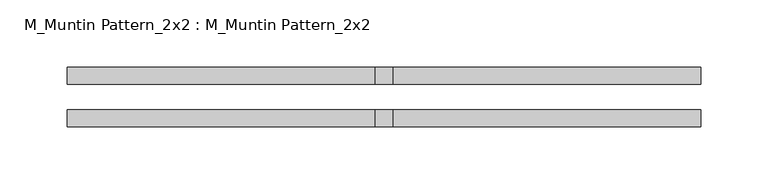
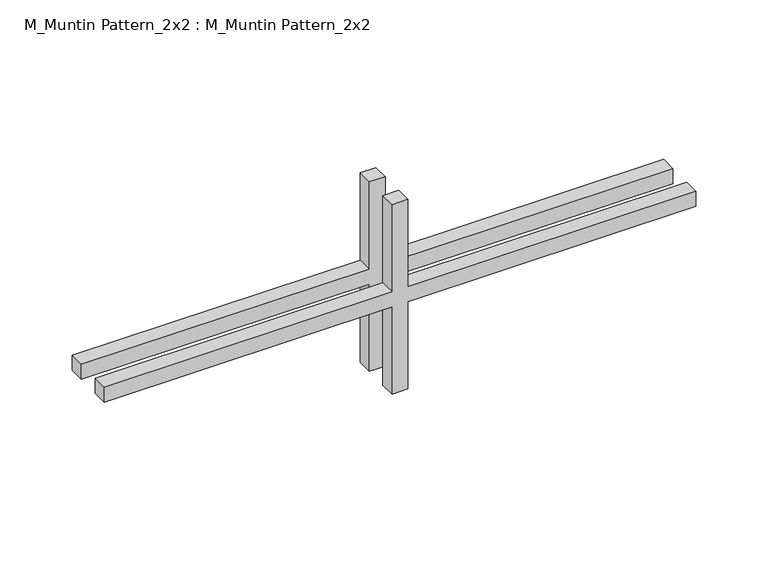
"""IFC4 building model written with IfcOpenShell, lengths in millimetres: proxy geometry, M_Muntin Pattern_2x2 : M_Muntin Pattern_2x2."""

from ifc_helpers import new_model, si_unit, frame, origin, place, context, project, spatial, polyline, outline, extrude, source, transform, mapped, element, save


def m_muntin_pattern_2x2_m_muntin_pattern_2x2_383df7b3(model_context):
    return source(origin(), model_context, "Body", "SweptSolid", [
        extrude(outline(polyline([(86.5, -6.35), (86.5, -236.5375), (73.8, -236.5375), (73.8, -6.35), (0.0, -6.35), (0.0, 6.35), (73.8, 6.35), (73.8, 236.5375), (86.5, 236.5375), (86.5, 6.35), (160.3, 6.35), (160.3, -6.35), (86.5, -6.35)])), frame((0.0, -22.225, 0.0), z_axis=(0.0, 1.0, 0.0), x_axis=(0.0, 0.0, 1.0)), (0.0, 0.0, 1.0), 12.7),
        extrude(outline(polyline([(86.5, -6.35), (86.5, -236.5375), (73.8, -236.5375), (73.8, -6.35), (0.0, -6.35), (0.0, 6.35), (73.8, 6.35), (73.8, 236.5375), (86.5, 236.5375), (86.5, 6.35), (160.3, 6.35), (160.3, -6.35), (86.5, -6.35)])), frame((0.0, 9.525, 0.0), z_axis=(0.0, 1.0, 0.0), x_axis=(0.0, 0.0, 1.0)), (0.0, 0.0, 1.0), 12.7),
    ])


if __name__ == "__main__":
    model = new_model("IFC4")
    model_context = context("Model", 3, world=origin())
    ifc_project = project(units=[si_unit("LENGTHUNIT", "METRE", prefix="MILLI")], contexts=[model_context])
    site = spatial("IfcSite", under=ifc_project)
    building = spatial("IfcBuilding", under=site)
    placement = place(None, origin())
    m_muntin_pattern_2x2_m_muntin_pattern_2x2_shape = m_muntin_pattern_2x2_m_muntin_pattern_2x2_383df7b3(model_context)
    element("IfcBuildingElementProxy", 1, Name="M_Muntin Pattern_2x2 : M_Muntin Pattern_2x2", ObjectType="M_Muntin Pattern_2x2 : M_Muntin Pattern_2x2", at=placement, inside=building, context=model_context, shape_type="MappedRepresentation", body=[
        mapped(m_muntin_pattern_2x2_m_muntin_pattern_2x2_shape, transform((0.0, 0.0, 0.0), x_axis=(1.0, 0.0, 0.0), y_axis=(0.0, 1.0, 0.0), z_axis=(0.0, 0.0, 1.0))),
    ])
    save(model, "model.ifc")

# Revit data of these elements
# Type "M_Muntin Pattern_2x2 : M_Muntin Pattern_2x2"
#   Width [instance default] = 3' - 11.24409"
#   Thickness = 0' - 0 1/2"
#   Height [instance default] = 3' - 11.24409"
#   Distance = 0' - 0 3/4"
#   Interior Material [instance default] = none
#   Exterior Material [instance default] = none
#   Default Elevation = 0
# Element 1 (IfcBuildingElementProxy, "M_Muntin Pattern_2x2 : M_Muntin Pattern_2x2")
#   Width = 1' - 6 5/8"
#   Height = 0' - 6.31102"
#   Interior Material = Wood - Stained
#   Exterior Material = Clad - White
#   Materials on its faces: "Clad - White", "Wood - Stained"
# Materials
#   "Clad - White": class "Wood", colour RGB 242 242 238, transparency 0, Cost = 0
#   "Wood - Stained": class "Wood", colour RGB 227 170 128, transparency 0, Cost = 0
